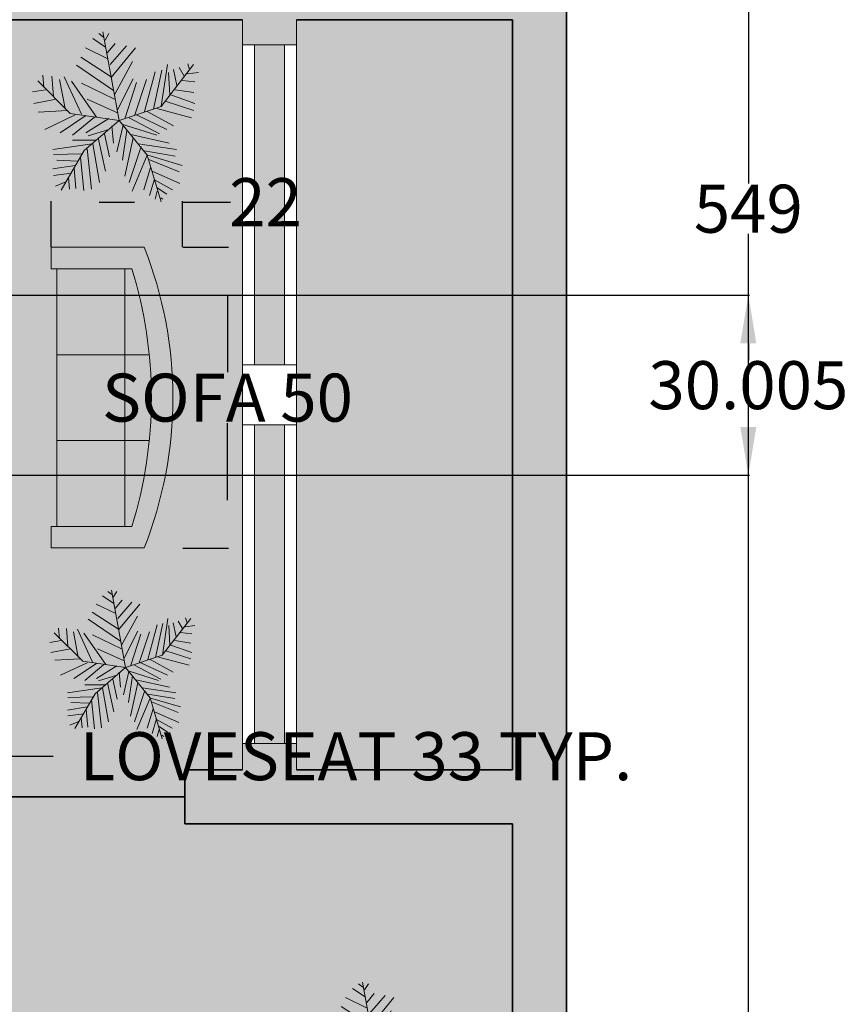
# Model space of a CAD drawing. Units: inches. Extents: x 389 to 971, y 148 to 870.
# Tile 13 of 14: x 757 to 895, y 428 to 592. Entities that reach past the tile are written whole.
import ezdxf

# ---------------------------------------------------------------- set-up
doc = ezdxf.new("R2010")
doc.units = ezdxf.units.IN
doc.header["$MEASUREMENT"] = 0
for name, color, linetype, lineweight in [('A-ANNO-DIMS', 2, 'Continuous', 18), ('A-FLOR-BASE-PATT', 8, 'Continuous', 13), ('A-FURN', 8, 'Continuous', 18), ('A-GLAZ', 4, 'Continuous', 18), ('A-WALL', 7, 'Continuous', 35), ('C-PROP', 7, 'Continuous', 35), ('L-GRND-BASE-PATT', 8, 'Continuous', 13), ('L-PLNT', 3, 'Continuous', 13)]:
    doc.layers.add(name, color=color, linetype=linetype, lineweight=lineweight)
for name, color, linetype, lineweight, true_color in [('A-FURN-SURF-PATT', 9, 'Continuous', 13, 0xd6bdce), ('A-GLAZ-PATT', 251, 'Continuous', 13, 0x6d5f6c), ('A-WALL-PATT', 18, 'Continuous', 13, 0x000000), ('L-GRND-PATT', 39, 'Continuous', 13, 0x603913)]:
    doc.layers.add(name, color=color, linetype=linetype, lineweight=lineweight, true_color=true_color)
doc.styles.get("Standard").update_dxf_attribs({"font": 'arial.ttf'})
doc.dimstyles.get("Standard").update_dxf_attribs({"dimtxt": 8, "dimasz": 8, "dimexe": 0.18, "dimexo": 0.0625, "dimgap": 0.09, "dimtad": 0, "dimtih": 1, "dimtoh": 1, "dimdec": 0, "dimzin": 0, "dimdsep": 46, "dimlunit": 3, "dimtxsty": 'Standard', "dimcen": 0.09, "dimadec": 0, "dimazin": 0, "dimtfac": 1, "dimtdec": 0, "dimtofl": 0, "dimtmove": 0, "dimatfit": 3, "dimfxl": 1, "dimtolj": 1, "dimtzin": 0, "dimarcsym": 0})

# ---------------------------------------------------------------- blocks, each defined once
blk = doc.blocks.new('Sofa - Roundback 7 ft.')
for p, q in [((-12.00002, -32.4421), (-12.00003, -6.5971)), ((11.99997, -32.4421), (11.99998, -6.5971)), ((-36.000027, -34), (-36.000027, -11.4696)), ((-35.999844, -13.3819), (35.9998, -13.3819)), ((35.99998, -34), (35.99998, -11.4696)), ((-36.000027, -32.4421), (35.99998, -32.4421))]:
    blk.add_line(p, q)
for points in [[(-36.000027, -34), (-42.000027, -34), (-42.000027, -8)], [(41.99998, -8), (41.99998, -34), (35.99998, -34)]]:
    blk.add_lwpolyline(points)
for centre, radius, start, end in [((0, -114.25), 114.25, 68.43141, 111.5686), ((-0.00001, -127.1968), 121.1968, 72.72033, 107.2797)]:
    blk.add_arc(centre, radius, start, end)
blk = doc.blocks.new('*U19')
for p, q in [((-221.9198, 1197.3052), (-433.5526, 1338.8594)), ((-258.7244, 1362.456), (-332.3336, 1421.4348)), ((0, 0), (-266.7, 1447.8)), ((-231.1146, 1315.2628), (-166.7002, 1421.4348)), ((-185.1152, 1008.5578), (-553.1612, 1185.4942)), ((-194.31, 1102.9442), (-65.4812, 1256.284)), ((-148.3106, 914.1968), (118.5418, 1220.9018)), ((-129.8956, 701.8528), (265.7602, 1185.4942)), ((-129.8956, 713.6638), (-626.7704, 1032.1544)), ((-93.091, 489.5342), (-700.3796, 902.3858)), ((-74.7014, 418.7444), (219.7608, 961.39)), ((560.197, 182.8292), (698.2206, 819.8358)), ((685.8, 228.6), (1219.2, 914.4)), ((689.0258, 230.0224), (790.2448, 914.1968)), ((891.4384, 831.6214), (946.658, 572.1096)), ((983.4626, 867.0036), (1066.2666, 725.4494)), ((1121.4862, 925.9824), (1149.0706, 831.6214)), ((-800.1, 114.3), (-1333.5, 647.7)), ((-1234.059, 536.7274), (-1252.4486, 737.2604)), ((-1105.2302, 725.4494), (-1077.6458, 395.1732)), ((-976.4268, 666.4706), (-884.4026, 194.6402)), ((-902.8176, 713.6638), (-617.5756, 100.2538)), ((-28.6766, 171.0436), (228.9556, 678.2816)), ((256.5654, 88.4682), (449.7832, 666.4706)), ((412.9786, 147.447), (587.8068, 796.2392)), ((808.6344, 784.4282), (827.0494, 418.7444)), ((1029.462, 654.685), (1241.0948, 631.0884)), ((1112.2914, 760.8316), (1296.3144, 784.4282)), ((-1206.4492, 501.3198), (-1418.082, 465.9376)), ((-369.1382, 53.086), (-783.1836, 642.874)), ((-617.5756, 607.4918), (-74.7014, 347.98)), ((100.1268, 41.275), (284.1498, 619.2774)), ((919.0482, 501.3198), (1222.6798, 454.152)), ((-1031.621, 347.98), (-1399.667, 277.1902)), ((-525.5514, 347.98), (-28.6766, 123.8504)), ((845.439, 418.7444), (1241.0948, 277.1902)), ((0, 0), (685.8, 228.6)), ((615.4166, 194.6402), (1185.8752, 41.275)), ((753.4148, 312.5978), (1222.6798, 159.2326)), ((-847.598, 159.2326), (-1326.0578, 135.636)), ((-718.7946, 88.4682), (-1215.644, -147.447)), ((-543.9664, 76.6572), (-967.2066, -206.4512)), ((0, 0), (-800.1, 114.3)), ((-405.9428, 53.086), (-764.794, -241.8334)), ((0, 0), (-571.5, -495.3)), ((-166.7002, 29.4894), (-543.9664, -206.4512)), ((0, 0), (457.2, -571.5)), ((164.5412, 41.275), (661.416, -218.2368)), ((284.1498, 88.4682), (781.0246, -147.447)), ((458.978, 147.447), (891.4384, -88.4682)), ((-166.7002, -147.447), (-507.1618, -253.619)), ((-120.7008, -88.4682), (-93.091, -371.5766)), ((63.3222, -76.6826), (-37.8714, -513.1308)), ((44.9326, -64.897), (615.4166, -241.8334)), ((127.7366, -159.258), (54.1274, -654.685)), ((-341.5284, -289.0012), (-221.9198, -831.6214)), ((-240.3094, -218.2368), (-157.5054, -595.7062)), ((228.9556, -289.0012), (90.932, -914.1968)), ((192.151, -230.0224), (817.8292, -371.5766)), ((-442.7474, -383.3876), (-1086.8406, -477.7486)), ((-387.5278, -324.4088), (-764.794, -324.4088)), ((-525.5514, -465.963), (-451.9422, -1126.5408)), ((-433.5526, -383.3876), (-323.1134, -1020.3688)), ((357.759, -430.5554), (164.5412, -1020.3688)), ((311.7596, -383.3876), (937.4378, -477.7486)), ((-617.5756, -548.5384), (-1077.6458, -560.324)), ((-571.5, -495.3), (-952.5, -1143)), ((-635.9652, -607.5172), (-580.771, -1150.1374)), ((458.978, -572.1096), (210.5406, -1161.923)), ((412.9786, -501.3452), (919.0482, -583.9206)), ((457.2, -571.5), (685.8, -1333.5)), ((468.1982, -572.1096), (1029.462, -737.2604)), ((486.5878, -642.8994), (983.4626, -843.4324)), ((-718.7946, -737.2604), (-1086.8406, -796.2392)), ((-681.9646, -666.496), (-1022.4262, -654.685)), ((-737.1842, -784.4536), (-709.5744, -1114.7298)), ((514.1976, -772.6426), (403.7838, -1138.3264)), ((-783.1836, -867.029), (-1077.6458, -902.4112)), ((-829.2084, -937.7934), (-810.7934, -1126.5408)), ((578.612, -961.39), (495.7826, -1232.7128)), ((541.8074, -831.6214), (992.6574, -1032.1544)), ((-875.2078, -1008.5832), (-1040.8412, -1079.3476)), ((578.612, -973.1756), (873.0488, -1138.3264)), ((624.6114, -1102.9442), (781.0246, -1209.1162)), ((624.6114, -1161.923), (587.8068, -1291.6916)), ((679.8056, -1268.095), (716.6102, -1291.6916))]:
    blk.add_line(p, q)
blk = doc.blocks.new('*D36')
at = {"layer": 'A-ANNO-DIMS', "color": 0, "lineweight": -2, "transparency": 16777216}
for p, q in [((784.27, 553.71), (791.91, 553.71)), ((791.73, 545.71), (791.73, 532.88)), ((791.73, 511.59), (791.73, 524.42)), ((784.27, 503.59), (791.91, 503.59))]:
    blk.add_line(p, q, dxfattribs=at)
at = {"layer": 'A-ANNO-DIMS', "color": 0, "transparency": 16777216}
for points in [[(790.39, 545.71), (793.06, 545.71), (791.73, 553.71)], [(790.39, 511.59), (793.06, 511.59), (791.73, 503.59)]]:
    blk.add_solid(points, dxfattribs=at)
at = {"layer": 'Defpoints', "color": 0, "transparency": 16777216}
for p in [(784.21, 553.71), (784.21, 503.59), (791.73, 503.59)]:
    blk.add_point(p, dxfattribs=at)
at = {"layer": 'A-ANNO-DIMS', "color": 0, "transparency": 16777216, "insert": (791.73, 528.65), "char_height": 8, "attachment_point": 5}
blk.add_mtext('\\A1;SOFA 50', dxfattribs=at)
blk = doc.blocks.new('*D37')
at = {"layer": 'A-ANNO-DIMS', "color": 0, "lineweight": -2, "transparency": 16777216}
for p, q in [((762.33, 553.77), (762.33, 561.41)), ((784.21, 553.77), (784.21, 561.41)), ((770.33, 561.23), (776.21, 561.23)), ((784.21, 561.23), (792.21, 561.23))]:
    blk.add_line(p, q, dxfattribs=at)
at = {"layer": 'A-ANNO-DIMS', "color": 0, "transparency": 16777216}
for points in [[(770.33, 562.56), (770.33, 559.89), (762.33, 561.23)], [(776.21, 562.56), (776.21, 559.89), (784.21, 561.23)]]:
    blk.add_solid(points, dxfattribs=at)
at = {"layer": 'Defpoints', "color": 0, "transparency": 16777216}
for p in [(784.21, 561.23), (762.33, 553.71), (784.21, 553.71)]:
    blk.add_point(p, dxfattribs=at)
at = {"layer": 'A-ANNO-DIMS', "color": 0, "transparency": 16777216, "insert": (798.06, 561.23), "char_height": 8, "attachment_point": 5}
blk.add_mtext('\\A1;22', dxfattribs=at)
blk = doc.blocks.new('*D40')
at = {"layer": 'A-ANNO-DIMS', "color": 0, "lineweight": -2, "transparency": 16777216}
for p, q in [((721.8, 473.76), (721.8, 468.71)), ((754.7, 473.76), (754.7, 468.71)), ((729.8, 468.89), (746.7, 468.89)), ((754.7, 468.89), (762.7, 468.89))]:
    blk.add_line(p, q, dxfattribs=at)
at = {"layer": 'A-ANNO-DIMS', "color": 0, "transparency": 16777216}
for points in [[(729.8, 470.23), (729.8, 467.56), (721.8, 468.89)], [(746.7, 470.23), (746.7, 467.56), (754.7, 468.89)]]:
    blk.add_solid(points, dxfattribs=at)
at = {"layer": 'Defpoints', "color": 0, "transparency": 16777216}
for p in [(721.8, 473.83), (754.7, 473.83), (754.7, 468.89)]:
    blk.add_point(p, dxfattribs=at)
at = {"layer": 'A-ANNO-DIMS', "color": 0, "transparency": 16777216, "insert": (813.14, 468.89), "char_height": 8, "attachment_point": 5}
blk.add_mtext('\\A1;LOVESEAT 33 TYP.', dxfattribs=at)
blk = doc.blocks.new('*D47')
at = {"layer": 'A-ANNO-DIMS', "color": 0, "lineweight": -2, "transparency": 16777216}
for p, q in [((848.28, 834.64), (878.72, 834.64)), ((878.54, 826.64), (878.54, 564.32)), ((878.54, 293.64), (878.54, 555.97)), ((839.28, 285.64), (878.72, 285.64))]:
    blk.add_line(p, q, dxfattribs=at)
at = {"layer": 'A-ANNO-DIMS', "color": 0, "transparency": 16777216}
for points in [[(877.21, 826.64), (879.87, 826.64), (878.54, 834.64)], [(877.21, 293.64), (879.87, 293.64), (878.54, 285.64)]]:
    blk.add_solid(points, dxfattribs=at)
at = {"layer": 'Defpoints', "color": 0, "transparency": 16777216}
for p in [(848.22, 834.64), (878.54, 834.64), (839.22, 285.64)]:
    blk.add_point(p, dxfattribs=at)
at = {"layer": 'A-ANNO-DIMS', "color": 0, "transparency": 16777216, "insert": (878.54, 560.14), "char_height": 8, "attachment_point": 5}
blk.add_mtext('\\A1;549', dxfattribs=at)
blk = doc.blocks.new('*D48')
at = {"layer": 'A-ANNO-DIMS', "color": 0, "lineweight": -2, "transparency": 16777216}
for p, q in [((595.45, 545.73), (878.72, 545.73)), ((878.54, 537.73), (878.54, 534.91)), ((878.54, 523.73), (878.54, 526.55)), ((595.45, 515.73), (878.72, 515.73))]:
    blk.add_line(p, q, dxfattribs=at)
at = {"layer": 'A-ANNO-DIMS', "color": 0, "transparency": 16777216}
for points in [[(877.21, 537.73), (879.87, 537.73), (878.54, 545.73)], [(877.21, 523.73), (879.87, 523.73), (878.54, 515.73)]]:
    blk.add_solid(points, dxfattribs=at)
at = {"layer": 'Defpoints', "color": 0, "transparency": 16777216}
for p in [(595.39, 545.73), (878.54, 545.73), (595.39, 515.73)]:
    blk.add_point(p, dxfattribs=at)
at = {"layer": 'A-ANNO-DIMS', "color": 0, "transparency": 16777216, "insert": (878.54, 530.73), "char_height": 8, "attachment_point": 5}
blk.add_mtext('\\A1;30.005', dxfattribs=at)

msp = doc.modelspace()

# ---------------------------------------------------------------- hatches: boundary and pattern name
at = {"layer": 'A-FLOR-BASE-PATT'}
h = msp.add_hatch(color=256, dxfattribs=at)
h.dxf.hatch_style = 1
h.paths.add_polyline_path([(634.6594, 428.4021), (634.6594, 427.0792), (634.6305, 427.0792, -0.40145271), (604.4225, 398.1652), (604.0817, 398.1199, -0.40145271), (632.0195, 371.3788), (632.0462, 371.3788), (632.0462, 370.1554), (604.387, 370.1554), (604.387, 366.7191), (640.0296, 366.7191), (640.0296, 321.4969, 1), (647.061, 321.4969), (647.061, 412.9189), (690.216, 412.9189), (690.216, 416.0006), (694.716, 416.0006), (702.2145, 416.0006, 0.39601219), (737.1392, 448.8066), (702.2145, 448.8066), (702.2145, 450.9936), (694.716, 450.9936), (690.216, 450.9936), (690.216, 466.6012), (708.7881, 466.6012), (708.7881, 462.1012), (784.6145, 462.1012), (784.6145, 466.6012), (794.216, 466.6012), (794.216, 591.6445), (708.5171, 591.6445), (708.5171, 596.1445), (708.5171, 602.9755, 0.39601219), (678.6314, 634.7912), (678.6314, 602.9755), (676.6391, 602.9755), (676.6391, 596.1445), (676.6391, 591.6445), (661.216, 591.6445), (661.216, 632.6445), (653.109, 632.6445), (653.109, 641.6445), (653.109, 642.1751), (651.6417, 642.1751), (651.6417, 675.6801, 0.40145271), (619.5719, 642.1751), (619.5719, 637.1445), (619.5147, 632.6445), (604.387, 632.6445), (604.387, 545.7317), (595.3894, 545.7317), (595.3894, 544.4199), (565.4338, 544.4199, 0.40145271), (595.3894, 515.7475), (599.887, 515.7475), (604.387, 515.7271), (604.387, 428.4021)])
h.paths.add_polyline_path([(721.8003, 493.9292), (725.0899, 493.9292), (725.0899, 493.075), (751.4065, 493.075), (751.4065, 493.9292), (754.6961, 493.9292), (754.6961, 479.6744, -0.26666697), (721.8003, 479.6744)], flags=16)
h.paths.add_polyline_path([(720.6421, 516.0583), (720.6421, 545.0393), (753.5806, 545.0393), (753.5806, 516.0583)], flags=16)
h.paths.add_polyline_path([(722.6421, 518.0583), (722.6421, 543.0393), (751.5806, 543.0393), (751.5806, 518.0583)], flags=0)
h.paths.add_polyline_path([(763.7396, 488.5801), (763.7822, 488.1156), (764.1436, 488.1761)], flags=16)
h.paths.add_polyline_path([(777.9011, 479.7417), (778.0475, 480.1886), (777.4745, 480.275)], flags=16)
h.paths.add_polyline_path([(762.3329, 503.5919), (762.3329, 507.1718), (763.2624, 507.1718), (763.2624, 550.1306), (762.3329, 550.1306), (762.3329, 553.7105), (777.8458, 553.7105, -0.19047621), (777.8458, 503.5919)], flags=16)
h.paths.add_polyline_path([(721.6097, 567.2898), (721.6097, 581.7362, -0.26666697), (754.9475, 581.7362), (754.9475, 567.2898), (751.6137, 567.2898), (751.6137, 568.1555), (724.9435, 568.1555), (724.9435, 567.2898)], flags=16)
h.paths.add_polyline_path([(774.6347, 521.4914), (774.6347, 535.811), (778.6837, 535.811, -0.04962821), (778.6837, 521.4914)], flags=0)
h.paths.add_polyline_path([(764.6624, 576.8996), (764.7454, 576.4742), (765.0717, 576.4903)], flags=16)
h.paths.add_polyline_path([(777.2772, 570.3652), (777.4444, 570.8756), (776.7899, 570.9743)], flags=16)
h.paths.add_polyline_path([(644.2892, 516.9956), (685.2491, 516.9956), (685.2491, 535.7223), (644.2892, 535.7223)], flags=24)
h = msp.add_hatch(color=256, dxfattribs=at)
h.dxf.hatch_style = 1
h.paths.add_polyline_path([(839.216, 591.6445), (803.216, 591.6445), (803.216, 466.6012), (839.216, 466.6012)])
h = msp.add_hatch(color=256, dxfattribs=at)
h.dxf.hatch_style = 1
h.paths.add_polyline_path([(699.216, 294.6445), (733.8057, 294.6445), (810.0514, 294.6445), (839.216, 294.6445), (839.216, 457.6012), (784.6145, 457.6012), (784.6145, 462.1012), (708.7881, 462.1012), (708.7881, 457.6012), (699.216, 457.6012), (699.216, 450.9936), (702.2145, 450.9936), (737.2076, 450.9936), (737.2076, 448.8066), (737.1392, 448.8066, -0.39601219), (702.2145, 416.0006), (699.216, 416.0006)])
h.paths.add_polyline_path([(755.1859, 373.9163), (788.1244, 373.9163), (788.1244, 344.9352), (755.1859, 344.9352)], flags=16)
h.paths.add_polyline_path([(757.1859, 371.9163), (786.1244, 371.9163), (786.1244, 346.9352), (757.1859, 346.9352)], flags=0)
h.paths.add_polyline_path([(746.1376, 327.3223), (750.14, 327.3223), (750.14, 326.2831), (798.1694, 326.2831), (798.1694, 327.3223), (802.1718, 327.3223), (802.1718, 309.9784, -0.19047621), (746.1376, 309.9784)], flags=16)
h.paths.add_polyline_path([(782.1596, 313.5685), (782.1596, 309.0415, -0.04962821), (766.1498, 309.0415), (766.1498, 313.5685)], flags=0)
h.paths.add_polyline_path([(804.6838, 390.5197), (803.6446, 390.5197), (803.6446, 394.5221), (820.9885, 394.5221, -0.19047621), (820.9885, 338.4879), (803.6446, 338.4879), (803.6446, 342.4903), (804.6838, 342.4903)], flags=16)
h.paths.add_polyline_path([(817.3984, 358.5001), (817.3984, 374.5099), (821.9254, 374.5099, -0.04962821), (821.9254, 358.5001)], flags=0)
h.paths.add_polyline_path([(806.8707, 326.6963), (806.4254, 327.1416), (806.4724, 326.6297)], flags=16)
h.paths.add_polyline_path([(822.0328, 317.4008), (822.1942, 317.8933), (821.5626, 317.9885)], flags=16)
h.paths.add_polyline_path([(808.1446, 418.9737), (808.2247, 418.5632), (808.5395, 418.5787)], flags=16)
h.paths.add_polyline_path([(820.3159, 412.669), (820.4772, 413.1615), (819.8457, 413.2568)], flags=16)
h.paths.add_polyline_path([(750.6082, 393.6667), (791.5681, 393.6667), (791.5681, 412.3933), (750.6082, 412.3933)], flags=24)
at = {"layer": 'A-FURN-SURF-PATT'}
h = msp.add_hatch(color=256, dxfattribs=at)
h.dxf.hatch_style = 1
h.paths.add_polyline_path([(777.8458, 553.7105), (762.3329, 553.7105), (762.3329, 550.1306), (775.7753, 550.1306, -0.15194781), (775.7753, 507.1718), (762.3329, 507.1718), (762.3329, 503.5919), (777.8458, 503.5919, 0.19047621)])
h = msp.add_hatch(color=256, dxfattribs=at)
h.dxf.hatch_style = 1
h.paths.add_polyline_path([(774.6347, 550.1306), (763.2624, 550.1306), (763.2624, 535.811), (774.6347, 535.811)])
h = msp.add_hatch(color=256, dxfattribs=at)
h.dxf.hatch_style = 1
h.paths.add_polyline_path([(775.7753, 550.1306), (774.6347, 550.1306), (774.6347, 535.811), (778.6837, 535.811, 0.05064665)])
h = msp.add_hatch(color=256, dxfattribs=at)
h.dxf.hatch_style = 1
h.paths.add_polyline_path([(763.2624, 521.4914), (774.6347, 521.4914), (774.6347, 535.811), (763.2624, 535.811)])
h = msp.add_hatch(color=256, dxfattribs=at)
h.dxf.hatch_style = 1
h.paths.add_polyline_path([(774.6347, 521.4914), (778.6837, 521.4914, 0.04962821), (778.6837, 535.811), (774.6347, 535.811)])
h = msp.add_hatch(color=256, dxfattribs=at)
h.dxf.hatch_style = 1
h.paths.add_polyline_path([(774.6347, 521.4914), (763.2624, 521.4914), (763.2624, 507.1718), (774.6347, 507.1718)])
h = msp.add_hatch(color=256, dxfattribs=at)
h.dxf.hatch_style = 1
h.paths.add_polyline_path([(774.6347, 507.1718), (775.7753, 507.1718, 0.05064665), (778.6837, 521.4914), (774.6347, 521.4914)])
at = {"layer": 'A-GLAZ-PATT'}
h = msp.add_hatch(color=256, dxfattribs=at)
h.dxf.hatch_style = 1
h.paths.add_polyline_path([(801.216, 587.4291), (796.216, 587.4291), (796.216, 534.1229), (801.216, 534.1229)])
h = msp.add_hatch(color=256, dxfattribs=at)
h.dxf.hatch_style = 1
h.paths.add_polyline_path([(796.216, 471.0309), (801.216, 471.0309), (801.216, 524.1229), (796.216, 524.1229)])
at = {"layer": 'A-WALL-PATT'}
h = msp.add_hatch(color=256, dxfattribs=at)
h.dxf.hatch_style = 1
h.paths.add_polyline_path([(432.216, 434.6445), (436.3673, 434.6445), (436.3673, 443.6445), (432.216, 443.6445), (432.216, 830.6445), (746.216, 830.6445), (746.216, 823.8175), (755.216, 823.8175), (755.216, 825.6445), (839.216, 825.6445), (839.216, 803.5176), (839.216, 741.6445), (755.216, 741.6445), (755.216, 748.4596), (755.1859, 748.4596), (750.716, 748.4596), (746.216, 748.4596), (746.216, 732.6445), (839.216, 732.6445), (839.216, 600.6445), (708.5171, 600.6445), (708.5171, 596.1445), (708.5171, 591.6445), (794.216, 591.6445), (794.216, 587.4291), (803.216, 587.4291), (803.216, 591.6445), (839.216, 591.6445), (839.216, 466.6012), (803.216, 466.6012), (803.216, 471.0309), (794.216, 471.0309), (794.216, 466.6012), (784.6145, 466.6012), (784.6145, 457.6012), (839.216, 457.6012), (839.216, 447.6445), (839.216, 294.6445), (810.0514, 294.6445), (810.0514, 285.6445), (839.216, 285.6445), (839.216, 238.6445), (590.216, 238.6445), (590.216, 234.6445), (848.216, 234.6445), (848.216, 834.6445), (428.216, 834.6445), (428.216, 234.6445), (437.216, 234.6445), (437.216, 243.6445), (432.216, 243.6445)])
at = {"layer": 'L-GRND-BASE-PATT'}
h = msp.add_hatch(color=256, dxfattribs=at)
h.dxf.hatch_style = 1
edge = h.paths.add_edge_path(flags=16)
edge.add_ellipse((8782.0026, 354.2473), major_axis=(-8296.9493, 0), ratio=0.84230387, start_angle=-0.09022909, end_angle=0.38386678, ccw=False)
edge.add_ellipse((485.0533, 368.2895), major_axis=(-1.1591, 0), ratio=0.84230387, start_angle=0, end_angle=90, ccw=False)
edge.add_line((483.8943, 368.2895), (483.8943, 387.6039))
edge.add_ellipse((485.0533, 387.2466), major_axis=(1.1591, 0), ratio=0.84230387, start_angle=90, end_angle=180, ccw=False)
edge.add_line((485.0533, 388.2229), (485.5047, 388.2229))
edge.add_ellipse((898.8202, 372.4897), major_axis=(413.7374, 0), ratio=0.84230387, start_angle=176.349572, end_angle=177.82005, ccw=False)
edge.add_ellipse((535.9119, 196.3855), major_axis=(-245.3972, 0), ratio=0.84230387, start_angle=-77.874034, end_angle=-76.219471, ccw=False)
edge.add_ellipse((535.9119, 201.7547), major_axis=(239.1274, 0), ratio=0.84230387, start_angle=100.209539, end_angle=102.444627, ccw=False)
edge.add_ellipse((473.3139, 564.9222), major_axis=(196.5637, 0), ratio=0.84230387, start_angle=-80.743434, end_angle=-77.445067)
edge.add_line((509.5535, 402.1941), (514.3535, 404.8483))
edge.add_line((514.3535, 404.8483), (514.3535, 404.7972))
edge.add_ellipse((514.3535, 404.2644), major_axis=(0.5795, 0), ratio=0.84230387, start_angle=52.06687, end_angle=90, ccw=False)
edge.add_line((514.6716, 404.6725), (519.1535, 402.1941))
edge.add_ellipse((555.3932, 564.9222), major_axis=(-196.5637, 0), ratio=0.84230387, start_angle=77.445067, end_angle=80.743434)
edge.add_ellipse((492.7951, 201.7547), major_axis=(239.1274, 0), ratio=0.84230387, start_angle=77.555373, end_angle=79.790461, ccw=False)
edge.add_ellipse((492.7951, 196.3855), major_axis=(245.3972, 0), ratio=0.84230387, start_angle=76.219471, end_angle=77.874034, ccw=False)
edge.add_ellipse((129.8868, 372.4897), major_axis=(-413.7374, 0), ratio=0.84230387, start_angle=182.17995, end_angle=183.650428, ccw=False)
edge.add_line((543.2023, 388.2229), (544.0779, 388.2229))
edge.add_ellipse((543.6537, 387.2466), major_axis=(-1.1591, 0), ratio=0.84230387, start_angle=180, end_angle=270, ccw=False)
edge.add_line((544.8128, 387.2466), (544.8128, 367.9322))
edge.add_ellipse((543.6537, 368.2895), major_axis=(1.1591, 0), ratio=0.84230387, start_angle=270, end_angle=360, ccw=False)
edge.add_ellipse((-7753.2956, 354.2473), major_axis=(-8296.9493, 0), ratio=0.84230387, start_angle=179.61613322, end_angle=180.09022909, ccw=False)
edge.add_line((543.3912, 298.6608), (544.0779, 298.6608))
edge.add_ellipse((543.6537, 297.6845), major_axis=(1.1591, 0), ratio=0.84230387, start_angle=0, end_angle=90, ccw=False)
edge.add_line((544.8128, 297.6845), (544.8128, 278.3701))
edge.add_ellipse((543.6537, 278.7275), major_axis=(-1.1591, 0), ratio=0.84230387, start_angle=90, end_angle=180, ccw=False)
edge.add_line((543.6537, 277.7512), (543.1566, 277.7512))
edge.add_ellipse((-7753.2956, 354.2473), major_axis=(-8296.9493, 0), ratio=0.84230387, start_angle=179.3813568, end_angle=179.47172853, ccw=False)
edge.add_ellipse((542.4236, 263.2763), major_axis=(-1.7386, 0), ratio=0.84230387, start_angle=179.371763, end_angle=248.464757, ccw=False)
edge.add_ellipse((-7753.8751, 354.2473), major_axis=(-8298.7403, 0), ratio=0.842303866, start_angle=179.35344592, end_angle=179.3717628, ccw=False)
edge.add_ellipse((540.0116, 260.6509), major_axis=(-4.1092, 0), ratio=0.84230387, start_angle=90, end_angle=179.353446, ccw=False)
edge.add_line((540.0116, 257.1897), (488.6954, 257.1897))
edge.add_ellipse((488.6954, 260.6509), major_axis=(4.1092, 0), ratio=0.84230387, start_angle=180.646554, end_angle=270, ccw=False)
edge.add_ellipse((8782.5821, 354.2473), major_axis=(-8298.7403, 0), ratio=0.842303872, start_angle=0.62823723, end_angle=0.64655411, ccw=False)
edge.add_ellipse((486.2834, 263.2763), major_axis=(-1.7386, 0), ratio=0.84230387, start_angle=-68.464756, end_angle=0.628237, ccw=False)
edge.add_ellipse((8782.0026, 354.2473), major_axis=(-8296.9493, 0), ratio=0.84230387, start_angle=0.52827147, end_angle=0.6465541, ccw=False)
edge.add_line((485.5504, 277.7512), (484.6291, 277.7512))
edge.add_ellipse((485.0533, 278.7275), major_axis=(-1.1591, 0), ratio=0.84230387, start_angle=0, end_angle=90, ccw=False)
edge.add_line((483.8943, 278.7275), (483.8943, 298.0418))
edge.add_ellipse((485.0533, 297.6845), major_axis=(1.1591, 0), ratio=0.84230387, start_angle=90, end_angle=180, ccw=False)
edge = h.paths.add_edge_path(flags=0)
edge.add_ellipse((8782.0026, 354.2473), major_axis=(-8295.7902, 0), ratio=0.84230387, start_angle=0.05559431, end_angle=0.37776419, ccw=False)
edge.add_line((486.2179, 346.1978), (489.3905, 335.8384))
edge.add_ellipse((3386.0114, 329.7263), major_axis=(-2896.63, 0), ratio=0.84230387, start_angle=-0.1208974, end_angle=0.3640763)
edge.add_line((489.4638, 311.3204), (486.4666, 299.5521))
edge = h.paths.add_edge_path(flags=0)
edge.add_ellipse((514.3535, 391.3731), major_axis=(-115.1513, 0), ratio=0.84230387, start_angle=76.401865, end_angle=103.598135)
edge.add_line((537.3428, 296.3333), (537.3428, 281.5897))
edge.add_ellipse((514.3535, 376.6295), major_axis=(-115.1513, 0), ratio=0.84230387, start_angle=76.401865, end_angle=103.598135, ccw=False)
edge.add_line((491.3643, 281.5897), (491.3643, 296.3333))
edge = h.paths.add_edge_path(flags=0)
edge.add_line((491.3643, 337.0752), (489.653, 349.9016))
edge.add_ellipse((510.1338, 298.7862), major_axis=(64.0481, 0), ratio=0.84230387, start_angle=94.277421, end_angle=111.834954, ccw=False)
edge.add_line((506.1068, 352.6274), (522.6002, 352.6274))
edge.add_ellipse((518.5732, 298.7862), major_axis=(64.0481, 0), ratio=0.84230387, start_angle=68.165046, end_angle=85.722579, ccw=False)
edge.add_line((539.0541, 349.9016), (537.3428, 337.0752))
edge.add_ellipse((516.5462, 287.5825), major_axis=(62.3305, 0), ratio=0.84230387, start_angle=67.208085, end_angle=85.12993)
edge.add_line((521.008, 339.949), (507.699, 339.949))
edge.add_ellipse((512.1609, 287.5825), major_axis=(62.3305, 0), ratio=0.84230387, start_angle=94.87007, end_angle=112.791915)
edge = h.paths.add_edge_path(flags=0)
edge.add_ellipse((493.6824, 273.9439), major_axis=(-2.3182, 0), ratio=0.84230387, start_angle=-90, end_angle=0, ccw=False)
edge.add_line((493.6824, 275.8965), (535.3743, 275.8965))
edge.add_ellipse((535.0246, 273.9439), major_axis=(2.3182, 0), ratio=0.84230387, start_angle=0, end_angle=90, ccw=False)
edge.add_line((537.3428, 273.9439), (537.3428, 258.6983))
edge.add_line((537.3428, 258.6983), (540.5912, 258.6983))
edge.add_ellipse((540.5912, 260.6509), major_axis=(-2.3182, 0), ratio=0.84230387, start_angle=90, end_angle=179.353446)
edge.add_line((540.5912, 258.6983), (487.7691, 258.6983))
edge.add_ellipse((488.1158, 260.6509), major_axis=(2.3182, 0), ratio=0.84230387, start_angle=180.646554, end_angle=270)
edge.add_line((488.1158, 258.6983), (491.3643, 258.6983))
edge.add_line((491.3643, 258.6983), (491.3643, 274.2384))
h.paths.add_polyline_path([(746.1376, 327.3223), (750.14, 327.3223), (750.14, 326.2831), (798.1694, 326.2831), (798.1694, 327.3223), (802.1718, 327.3223), (802.1718, 309.9784, -0.19047621), (746.1376, 309.9784)], flags=16)
h.paths.add_polyline_path([(782.1596, 313.5685), (782.1596, 309.0415, -0.04962821), (766.1498, 309.0415), (766.1498, 313.5685)], flags=0)
h.paths.add_polyline_path([(755.1859, 344.9352), (755.1859, 373.9163), (788.1244, 373.9163), (788.1244, 344.9352)], flags=16)
h.paths.add_polyline_path([(757.1859, 346.9352), (757.1859, 371.9163), (786.1244, 371.9163), (786.1244, 346.9352)], flags=0)
h.paths.add_polyline_path([(803.6446, 338.4879), (803.6446, 342.4903), (804.6838, 342.4903), (804.6838, 390.5197), (803.6446, 390.5197), (803.6446, 394.5221), (820.9885, 394.5221, -0.19047621), (820.9885, 338.4879)], flags=16)
h.paths.add_polyline_path([(806.8707, 326.6963), (806.4254, 327.1416), (806.4724, 326.6297)], flags=16)
h.paths.add_polyline_path([(822.0328, 317.4008), (822.1942, 317.8933), (821.5626, 317.9885)], flags=16)
h.paths.add_polyline_path([(817.3984, 358.5001), (817.3984, 374.5099), (821.9254, 374.5099, -0.04962821), (821.9254, 358.5001)], flags=0)
h.paths.add_polyline_path([(808.1446, 418.9737), (808.2247, 418.5632), (808.5395, 418.5787)], flags=16)
h.paths.add_polyline_path([(820.3159, 412.669), (820.4772, 413.1615), (819.8457, 413.2568)], flags=16)
h.paths.add_polyline_path([(466.3155, 235.5246), (517.3807, 235.5246), (517.3807, 244.4269), (466.3155, 244.4269)], flags=24)
h.paths.add_polyline_path([(739.8737, 256.2), (815.404, 256.2), (815.404, 265.3454), (739.8737, 265.3454)], flags=24)
h.paths.add_polyline_path([(750.6082, 393.6667), (791.5681, 393.6667), (791.5681, 412.3933), (750.6082, 412.3933)], flags=24)
h.paths.add_polyline_path([(438.9631, 410.0619), (484.6204, 410.0619), (484.6204, 429.1217), (438.9631, 429.1217)], flags=24)
edge = h.paths.add_edge_path()
edge.add_line((839.216, 285.6445), (611.8787, 285.6445))
edge.add_line((611.8787, 285.6445), (604.387, 285.6445))
edge.add_line((604.387, 285.6445), (595.387, 285.6445))
edge.add_line((595.387, 285.6445), (595.387, 370.1554))
edge.add_line((595.387, 370.1554), (604.0817, 370.1554))
edge.add_line((604.0817, 370.1554), (604.0817, 371.3788))
edge.add_line((604.0817, 371.3788), (632.0195, 371.3788))
edge.add_arc((604.0817, 370.1554), 27.9645, 2.507491, 90)
edge.add_line((604.0817, 398.1199), (599.887, 398.1652))
edge.add_line((599.887, 398.1652), (604.4225, 398.1652))
edge.add_arc((604.4225, 428.4021), 30.2369, 270, 357.492509)
edge.add_line((634.6305, 427.0792), (604.4225, 427.0792))
edge.add_line((604.4225, 427.0792), (604.4225, 428.4021))
edge.add_line((604.4225, 428.4021), (599.887, 428.4021))
edge.add_line((599.887, 428.4021), (595.387, 428.4021))
edge.add_line((595.387, 428.4021), (595.387, 434.6445))
edge.add_line((595.387, 434.6445), (585.0791, 434.6445))
edge.add_line((585.0791, 434.6445), (540.3922, 434.6445))
edge.add_line((540.3922, 434.6445), (526.7125, 434.6445))
edge.add_line((526.7125, 434.6445), (488.4095, 434.6445))
edge.add_line((488.4095, 434.6445), (432.216, 434.6445))
edge.add_line((432.216, 434.6445), (432.216, 243.6445))
edge.add_line((432.216, 243.6445), (437.216, 243.6445))
edge.add_line((437.216, 243.6445), (437.216, 234.6445))
edge.add_line((437.216, 234.6445), (581.216, 234.6445))
edge.add_line((581.216, 234.6445), (581.216, 238.6445))
edge.add_line((581.216, 238.6445), (581.216, 243.6445))
edge.add_line((581.216, 243.6445), (590.216, 243.6445))
edge.add_line((590.216, 243.6445), (590.216, 238.6445))
edge.add_line((590.216, 238.6445), (839.216, 238.6445))
edge.add_line((839.216, 238.6445), (839.216, 285.6445))
at = {"layer": 'L-GRND-PATT'}
h = msp.add_hatch(dxfattribs=at)
h.set_pattern_fill('EARTH', color=256, angle=45)
h.set_pattern_definition([(45, (0, 0), (0, 8.980256), [6.35, -6.35]), (45, (-1.684, 1.684), (0, 8.980256), [6.35, -6.35]), (45, (-3.3676, 3.3676), (0, 8.980256), [6.35, -6.35]), (135, (-3.3676, 4.49), (-8.980256, 0), [6.35, -6.35]), (135, (-1.684, 6.174), (-8.980256, 0), [6.35, -6.35]), (135, (0, 7.858), (-8.980256, 0), [6.35, -6.35])])
h.paths.add_polyline_path([(432.216, 243.6445), (437.216, 243.6445), (437.216, 234.6445), (581.216, 234.6445), (581.216, 238.6445), (581.216, 243.6445), (590.216, 243.6445), (590.216, 238.6445), (839.216, 238.6445), (839.216, 285.6445), (810.0514, 285.6445), (733.8057, 285.6445), (684.2434, 285.6445), (611.8787, 285.6445), (604.387, 285.6445), (595.387, 285.6445), (595.387, 370.1554), (604.0817, 370.1554), (604.0817, 371.3788), (632.0195, 371.3788, 0.40145271), (604.0817, 398.1199), (599.887, 398.1652), (604.4225, 398.1652, 0.40145271), (634.6305, 427.0792), (604.4225, 427.0792), (604.4225, 428.4021), (599.887, 428.4021), (595.387, 428.4021), (595.387, 434.6445), (585.0791, 434.6445), (540.3922, 434.6445), (526.7125, 434.6445), (488.4095, 434.6445), (432.216, 434.6445)])
edge = h.paths.add_edge_path(flags=16)
edge.add_line((483.8943, 278.7275), (483.8943, 298.2564))
edge.add_ellipse((485.0533, 297.6845), major_axis=(1.1591, 0), ratio=0.84230387, start_angle=90, end_angle=180, ccw=False)
edge.add_ellipse((8782.0026, 354.2473), major_axis=(-8296.9493, 0), ratio=0.84230387, start_angle=-0.09022909, end_angle=0.38386678, ccw=False)
edge.add_ellipse((485.0533, 368.2895), major_axis=(-1.1591, 0), ratio=0.84230387, start_angle=0, end_angle=90, ccw=False)
edge.add_line((483.8943, 368.2895), (483.8943, 387.8185))
edge.add_ellipse((485.0533, 387.2466), major_axis=(1.1591, 0), ratio=0.84230387, start_angle=90, end_angle=180, ccw=False)
edge.add_ellipse((898.8202, 372.4897), major_axis=(413.7374, 0), ratio=0.84230387, start_angle=176.349572, end_angle=177.82005, ccw=False)
edge.add_ellipse((535.9119, 196.3855), major_axis=(-245.3972, 0), ratio=0.84230387, start_angle=-77.874034, end_angle=-76.219471, ccw=False)
edge.add_ellipse((535.9119, 201.7547), major_axis=(239.1274, 0), ratio=0.84230387, start_angle=100.209539, end_angle=102.444627, ccw=False)
edge.add_ellipse((473.3139, 564.9222), major_axis=(196.5637, 0), ratio=0.84230387, start_angle=-80.743434, end_angle=-77.445067)
edge.add_line((509.5535, 402.1941), (514.3535, 404.8483))
edge.add_line((514.3535, 404.8483), (519.1535, 402.1941))
edge.add_ellipse((555.3932, 564.9222), major_axis=(-196.5637, 0), ratio=0.84230387, start_angle=77.445067, end_angle=80.743434)
edge.add_ellipse((492.7951, 201.7547), major_axis=(239.1274, 0), ratio=0.84230387, start_angle=77.555373, end_angle=79.790461, ccw=False)
edge.add_ellipse((492.7951, 196.3855), major_axis=(245.3972, 0), ratio=0.84230387, start_angle=76.219471, end_angle=77.874034, ccw=False)
edge.add_ellipse((129.8868, 372.4897), major_axis=(-413.7374, 0), ratio=0.84230387, start_angle=182.17995, end_angle=183.650428, ccw=False)
edge.add_line((543.2023, 388.2229), (544.3327, 388.2229))
edge.add_ellipse((543.6537, 387.2466), major_axis=(-1.1591, 0), ratio=0.84230387, start_angle=180, end_angle=270, ccw=False)
edge.add_line((544.8128, 387.2466), (544.8128, 367.7176))
edge.add_ellipse((543.6537, 368.2895), major_axis=(1.1591, 0), ratio=0.84230387, start_angle=270, end_angle=360, ccw=False)
edge.add_ellipse((-7753.2956, 354.2473), major_axis=(-8296.9493, 0), ratio=0.84230387, start_angle=179.61613322, end_angle=180.09022909, ccw=False)
edge.add_ellipse((543.6537, 297.6845), major_axis=(1.1591, 0), ratio=0.84230387, start_angle=0, end_angle=90, ccw=False)
edge.add_line((544.8128, 297.6845), (544.8128, 278.1556))
edge.add_ellipse((543.6537, 278.7275), major_axis=(-1.1591, 0), ratio=0.84230387, start_angle=90, end_angle=180, ccw=False)
edge.add_ellipse((-7753.2956, 354.2473), major_axis=(-8296.9493, 0), ratio=0.84230387, start_angle=179.3813568, end_angle=179.47172853, ccw=False)
edge.add_ellipse((542.4236, 263.2763), major_axis=(-1.7386, 0), ratio=0.84230387, start_angle=179.371763, end_angle=248.464757, ccw=False)
edge.add_ellipse((-7753.8751, 354.2473), major_axis=(-8298.7403, 0), ratio=0.842303866, start_angle=179.35344592, end_angle=179.3717628, ccw=False)
edge.add_ellipse((540.0116, 260.6509), major_axis=(-4.1092, 0), ratio=0.84230387, start_angle=90, end_angle=179.353446, ccw=False)
edge.add_line((540.0116, 257.1897), (488.0808, 257.1897))
edge.add_ellipse((488.6954, 260.6509), major_axis=(4.1092, 0), ratio=0.84230387, start_angle=180.646554, end_angle=270, ccw=False)
edge.add_ellipse((8782.5821, 354.2473), major_axis=(-8298.7403, 0), ratio=0.842303872, start_angle=0.62823723, end_angle=0.64655411, ccw=False)
edge.add_ellipse((486.2834, 263.2763), major_axis=(-1.7386, 0), ratio=0.84230387, start_angle=-68.464756, end_angle=0.628237, ccw=False)
edge.add_ellipse((8782.0026, 354.2473), major_axis=(-8296.9493, 0), ratio=0.84230387, start_angle=0.52827147, end_angle=0.6465541, ccw=False)
edge.add_line((485.5504, 277.7512), (484.3744, 277.7512))
edge.add_ellipse((485.0533, 278.7275), major_axis=(-1.1591, 0), ratio=0.84230387, start_angle=0, end_angle=90, ccw=False)
edge = h.paths.add_edge_path(flags=0)
edge.add_ellipse((488.1158, 260.6509), major_axis=(2.3182, 0), ratio=0.84230387, start_angle=180.646554, end_angle=270)
edge.add_line((488.1158, 258.6983), (491.3643, 258.6983))
edge.add_line((491.3643, 258.6983), (491.3643, 274.4686))
edge.add_ellipse((493.6824, 273.9439), major_axis=(-2.3182, 0), ratio=0.84230387, start_angle=-90, end_angle=0, ccw=False)
edge.add_line((493.6824, 275.8965), (535.6476, 275.8965))
edge.add_ellipse((535.0246, 273.9439), major_axis=(2.3182, 0), ratio=0.84230387, start_angle=0, end_angle=90, ccw=False)
edge.add_line((537.3428, 273.9439), (537.3428, 258.6983))
edge.add_line((537.3428, 258.6983), (541.2086, 258.6983))
edge.add_ellipse((540.5912, 260.6509), major_axis=(-2.3182, 0), ratio=0.84230387, start_angle=90, end_angle=179.353446, ccw=False)
edge.add_line((540.5912, 258.6983), (487.4984, 258.6983))
edge = h.paths.add_edge_path(flags=0)
edge.add_line((491.3643, 281.5897), (491.3643, 296.3333))
edge.add_ellipse((514.3535, 391.3731), major_axis=(-115.1513, 0), ratio=0.84230387, start_angle=76.401865, end_angle=103.598135)
edge.add_line((537.3428, 296.3333), (537.3428, 281.5897))
edge.add_ellipse((514.3535, 376.6295), major_axis=(-115.1513, 0), ratio=0.84230387, start_angle=76.401865, end_angle=103.598135, ccw=False)
edge = h.paths.add_edge_path(flags=0)
edge.add_ellipse((8782.0026, 354.2473), major_axis=(-8295.7902, 0), ratio=0.84230387, start_angle=0.05559431, end_angle=0.37776419, ccw=False)
edge.add_line((486.2179, 346.1978), (489.3905, 335.8384))
edge.add_ellipse((3386.0114, 329.7263), major_axis=(-2896.63, 0), ratio=0.84230387, start_angle=-0.1208974, end_angle=0.3640763)
edge.add_line((489.4638, 311.3204), (486.4666, 299.5521))
edge = h.paths.add_edge_path(flags=0)
edge.add_line((491.3643, 337.0752), (489.653, 349.9016))
edge.add_ellipse((510.1338, 298.7862), major_axis=(64.0481, 0), ratio=0.84230387, start_angle=94.277421, end_angle=111.834954, ccw=False)
edge.add_line((506.1068, 352.6274), (522.6002, 352.6274))
edge.add_ellipse((518.5732, 298.7862), major_axis=(64.0481, 0), ratio=0.84230387, start_angle=68.165046, end_angle=85.722579, ccw=False)
edge.add_line((539.0541, 349.9016), (537.3428, 337.0752))
edge.add_ellipse((516.5462, 287.5825), major_axis=(62.3305, 0), ratio=0.84230387, start_angle=67.208085, end_angle=85.12993)
edge.add_line((521.008, 339.949), (507.699, 339.949))
edge.add_ellipse((512.1609, 287.5825), major_axis=(62.3305, 0), ratio=0.84230387, start_angle=94.87007, end_angle=112.791915)
h.paths.add_polyline_path([(466.3155, 235.5246), (517.3807, 235.5246), (517.3807, 244.4269), (466.3155, 244.4269)], flags=24)
h.paths.add_polyline_path([(739.8737, 256.2), (815.404, 256.2), (815.404, 265.3454), (739.8737, 265.3454)], flags=24)
h.paths.add_polyline_path([(438.9631, 410.0619), (484.6204, 410.0619), (484.6204, 429.1217), (438.9631, 429.1217)], flags=24)

# ---------------------------------------------------------------- linework, layer by layer
at = {"layer": 'A-GLAZ'}
for p, q in [((794.216, 466.6012), (794.216, 591.6445)), ((803.216, 466.6012), (803.216, 591.6445)), ((794.216, 587.4291), (803.216, 587.4291)), ((796.216, 534.1229), (796.216, 587.4291)), ((801.216, 534.1229), (801.216, 587.4291)), ((803.216, 534.1229), (794.216, 534.1229)), ((794.216, 534.1229), (794.216, 524.1229)), ((803.216, 529.1229), (803.216, 534.1229)), ((794.216, 524.1229), (803.216, 524.1229)), ((796.216, 471.0309), (796.216, 524.1229)), ((801.216, 471.0309), (801.216, 524.1229)), ((794.216, 471.0309), (803.216, 471.0309))]:
    msp.add_line(p, q, dxfattribs=at)
at = {"layer": 'A-WALL'}
for p, q in [((794.216, 591.6445), (708.5171, 591.6445)), ((794.216, 591.6445), (746.216, 591.6445)), ((839.216, 591.6445), (803.216, 591.6445)), ((839.216, 466.6012), (839.216, 591.6445)), ((784.6145, 466.6012), (784.6145, 457.6012)), ((794.216, 466.6012), (784.6145, 466.6012)), ((839.216, 466.6012), (803.216, 466.6012)), ((784.6145, 462.1012), (708.7881, 462.1012)), ((839.216, 457.6012), (784.6145, 457.6012)), ((839.216, 447.6445), (839.216, 457.6012)), ((839.216, 294.6445), (839.216, 457.6012))]:
    msp.add_line(p, q, dxfattribs=at)
at = {"layer": 'C-PROP'}
msp.add_line((848.216, 234.6445), (848.216, 834.6445), dxfattribs=at)

# ---------------------------------------------------------------- block references
at = {"layer": 'A-FURN', "xscale": 0.5966493437204862, "yscale": 0.5966493437204862, "zscale": 0.5966493437204862, "rotation": 270}
msp.add_blockref('Sofa - Roundback 7 ft.', (782.619, 528.6512), dxfattribs=at)
at = {"layer": 'L-PLNT'}
for p, xscale, yscale, zscale in [((773.6749, 574.8682), 0.0101793576421732, 0.0101793576421732, 0.0101793576421732), ((774.7474, 483.6839), 0.0089115603915329, 0.0089115603915329, 0.0089115603915329), ((816.8402, 417.0137), 0.0098214307456944, 0.0098214307456944, 0.0098214307456944)]:
    msp.add_blockref('*U19', p, dxfattribs=dict(at, xscale=xscale, yscale=yscale, zscale=zscale))

# ---------------------------------------------------------------- dimensions: what is measured, and where the dimension line sits
at = {"layer": 'A-ANNO-DIMS'}
for base, p1, p2, override, picture, middle in [((878.541, 834.6445), (839.216, 285.6445), (848.216, 834.6445), {"dimdec": 0, "dimlfac": 1, "dimrnd": 0, "dimzin": 0, "dimdsep": 46, "dimlunit": 2}, '*D47', (878.541, 560.1445)), ((878.541, 545.7317), (595.387, 515.7271), (595.387, 545.7317), {"dimdec": 3, "dimlfac": 1, "dimrnd": 0, "dimzin": 0, "dimdsep": 46, "dimlunit": 2}, '*D48', (878.541, 530.7294))]:
    dim = msp.add_linear_dim(base=base, p1=p1, p2=p2, angle=90, dimstyle='Standard', override=override, dxfattribs=at)
    dim.commit()
    dim.dimension.update_dxf_attribs({"geometry": picture, "text_midpoint": middle})
dim = msp.add_linear_dim(base=(784.21, 561.2282), p1=(762.3329, 553.7105), p2=(784.21, 553.7105), dimstyle='Standard', override={"dimdec": 0, "dimlfac": 1, "dimrnd": 0, "dimzin": 0, "dimdsep": 46, "dimlunit": 2}, dxfattribs=at)
dim.commit()
dim.dimension.update_dxf_attribs({"geometry": '*D37', "text_midpoint": (798.0572, 561.2282)})
dim = msp.add_linear_dim(base=(791.7278, 503.5919), p1=(784.21, 553.7105), p2=(784.21, 503.5919), angle=270, text='SOFA <>', dimstyle='Standard', override={"dimdec": 0, "dimlfac": 1, "dimrnd": 0, "dimzin": 0, "dimdsep": 46, "dimlunit": 2}, dxfattribs=at)
dim.commit()
dim.dimension.update_dxf_attribs({"geometry": '*D36', "text_midpoint": (791.7278, 528.6512)})
dim = msp.add_linear_dim(base=(754.6961, 468.8918), p1=(721.8003, 473.8262), p2=(754.6961, 473.8262), text='LOVESEAT <> TYP.', dimstyle='Standard', override={"dimdec": 0, "dimlfac": 1, "dimrnd": 0, "dimzin": 0, "dimdsep": 46, "dimlunit": 2}, dxfattribs=at)
dim.commit()
dim.dimension.update_dxf_attribs({"geometry": '*D40', "text_midpoint": (813.1354, 468.8918)})

doc.saveas('drawing.dxf')
